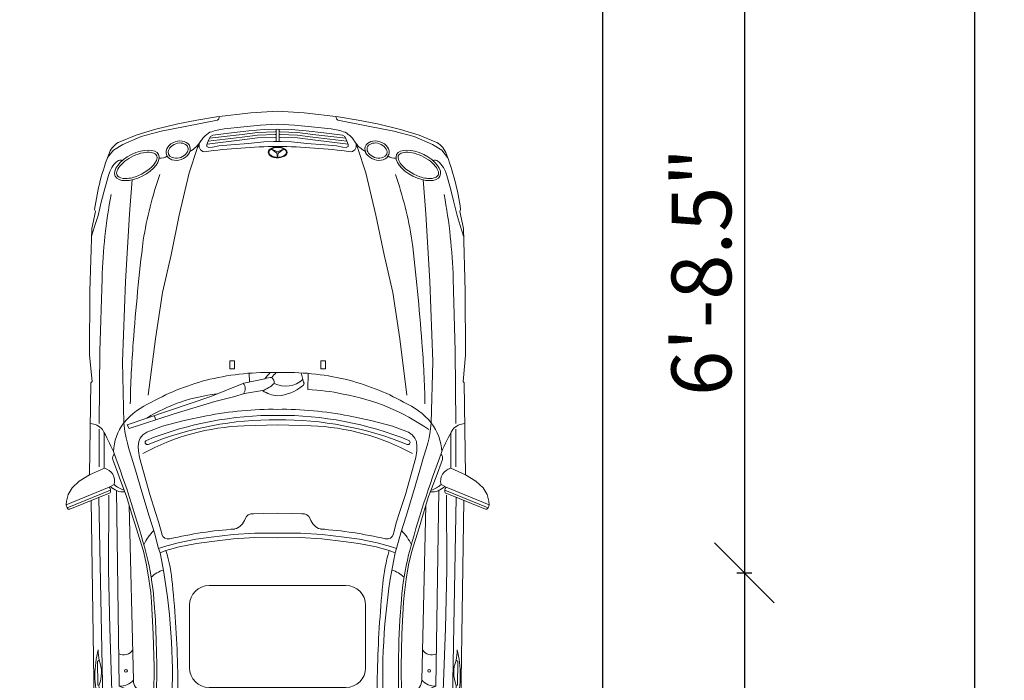
# Model space of a CAD drawing. Units: inches. Extents: x 2561 to 3163, y 493 to 1211.
# Tile 5 of 8: x 3031 to 3163, y 600 to 689. Entities that reach past the tile are written whole.
import ezdxf

# ---------------------------------------------------------------- set-up
doc = ezdxf.new("R2010")
doc.units = ezdxf.units.IN
for name, color, linetype, lineweight in [('0_Equip', 250, 'Continuous', 13), ('A-ANNO-DIMS', 2, 'Continuous', 18), ('A-SITE-PRKG', 8, 'Continuous', 25)]:
    doc.layers.add(name, color=color, linetype=linetype, lineweight=lineweight)
doc.styles.get("Standard").update_dxf_attribs({"font": 'arial.ttf'})
doc.dimstyles.new('ISO-25', dxfattribs={"dimtxt": 8, "dimasz": 8, "dimexe": 1, "dimexo": 1, "dimtad": 1, "dimlunit": 3, "dimtxsty": 'Standard', "dimblk": 'OBLIQUE', "dimcen": 2.5, "dimadec": 0, "dimazin": 0, "dimtfac": 1, "dimtmove": 0, "dimatfit": 3, "dimfxl": 1, "dimfxlon": 1, "dimarcsym": 0})

# ---------------------------------------------------------------- blocks, each defined once
blk = doc.blocks.new('A$C4C7B54D1')
at = {"layer": '0_Equip', "ltscale": 0.1}
for p, q in [((-1.0176, 2.6505), (-1.112, 2.6343)), ((-0.8531, 2.6707), (-1.0176, 2.6505)), ((-0.7257, 2.678), (-0.8531, 2.6707)), ((-0.7257, 2.678), (-0.5983, 2.6707)), ((-0.5983, 2.6707), (-0.4338, 2.6505)), ((-0.4338, 2.6505), (-0.3394, 2.6343)), ((-1.2037, 2.6168), (-1.3142, 2.5898)), ((-1.1673, 2.6045), (-1.2824, 2.5829)), ((-1.112, 2.6343), (-1.2037, 2.6168)), ((-1.0138, 2.6343), (-1.1673, 2.6045)), ((-0.8877, 2.6027), (-0.9812, 2.5937)), ((-0.8072, 2.6112), (-0.8877, 2.6027)), ((-0.7257, 2.6157), (-0.8072, 2.6112)), ((-0.7257, 2.6157), (-0.6441, 2.6112)), ((-0.6441, 2.6112), (-0.5636, 2.6027)), ((-0.5636, 2.6027), (-0.4701, 2.5937)), ((-0.4376, 2.6343), (-0.284, 2.6045)), ((-0.3394, 2.6343), (-0.2477, 2.6168)), ((-0.284, 2.6045), (-0.1689, 2.5829)), ((-0.2477, 2.6168), (-0.1371, 2.5898)), ((-1.4032, 2.5628), (-1.4801, 2.5318)), ((-1.3789, 2.557), (-1.4667, 2.5181)), ((-1.3142, 2.5898), (-1.4032, 2.5628)), ((-1.2824, 2.5829), (-1.3789, 2.557)), ((-0.1689, 2.5829), (-0.0725, 2.557)), ((-0.1371, 2.5898), (-0.0481, 2.5628)), ((-0.0725, 2.557), (0.0153, 2.5181)), ((-0.0481, 2.5628), (0.0288, 2.5318)), ((-1.4667, 2.5181), (-1.5113, 2.4907)), ((-1.1083, 2.5037), (-1.1486, 2.3827)), ((-0.343, 2.5037), (-0.3027, 2.3827)), ((0.0153, 2.5181), (0.06, 2.4907)), ((-1.5113, 2.4907), (-1.5393, 2.4562)), ((0.06, 2.4907), (0.0879, 2.4562)), ((-1.5353, 2.3701), (-1.5529, 2.308)), ((-1.1486, 2.3827), (-1.1961, 2.1797)), ((-0.3027, 2.3827), (-0.2552, 2.1797)), ((0.084, 2.3701), (0.1016, 2.308)), ((-1.435, 2.1869), (-1.4221, 2.3511)), ((-0.0163, 2.1869), (-0.0293, 2.3511)), ((-1.5529, 2.308), (-1.5677, 2.2486)), ((0.1016, 2.308), (0.1164, 2.2486)), ((-1.5677, 2.2486), (-1.5849, 2.1795)), ((0.1164, 2.2486), (0.1336, 2.1795)), ((-1.597, 2.1976), (-1.615, 2.1169)), ((-1.6012, 2.2082), (-1.597, 2.1976)), ((-1.5849, 2.1795), (-1.5997, 2.1304)), ((-1.4537, 1.863), (-1.435, 2.1869)), ((-1.1961, 2.1797), (-1.2349, 1.9911)), ((-0.2552, 2.1797), (-0.2164, 1.9911)), ((0.0024, 1.863), (-0.0163, 2.1869)), ((0.1336, 2.1795), (0.1484, 2.1304)), ((0.1499, 2.2082), (0.1457, 2.1976)), ((0.1457, 2.1976), (0.1637, 2.1169)), ((-1.5997, 2.1304), (-1.6161, 2.0798)), ((0.1484, 2.1304), (0.1647, 2.0798)), ((-1.615, 2.1169), (-1.6235, 1.8165)), ((0.1637, 2.1169), (0.1722, 1.8165)), ((-1.2349, 1.9911), (-1.2767, 1.8097)), ((-0.2164, 1.9911), (-0.1746, 1.8097)), ((-1.566, 1.8774), (-1.5761, 1.5304)), ((-1.4681, 1.48), (-1.4537, 1.863)), ((0.0168, 1.48), (0.0024, 1.863)), ((0.1147, 1.8774), (0.1247, 1.5304)), ((-1.6235, 1.8165), (-1.6256, 1.5098)), ((-1.2767, 1.8097), (-1.3098, 1.588)), ((-0.1746, 1.8097), (-0.1415, 1.588)), ((0.1722, 1.8165), (0.1743, 1.5098)), ((-1.3098, 1.588), (-1.3443, 1.3187)), ((-0.1415, 1.588), (-0.107, 1.3187)), ((-1.6256, 1.5098), (-1.6129, 1.3846)), ((-1.5761, 1.5304), (-1.5789, 1.1834)), ((0.1247, 1.5304), (0.1276, 1.1834)), ((0.1743, 1.5098), (0.1616, 1.3846)), ((-1.461, 1.1868), (-1.4681, 1.48)), ((-0.955, 1.4459), (-0.955, 1.4827)), ((-0.955, 1.4827), (-0.9321, 1.4827)), ((-0.9321, 1.4827), (-0.9321, 1.4459)), ((-0.5192, 1.4827), (-0.5192, 1.4459)), ((-0.4964, 1.4827), (-0.5192, 1.4827)), ((-0.4964, 1.4459), (-0.4964, 1.4827)), ((0.0097, 1.1868), (0.0168, 1.48)), ((-0.9321, 1.4459), (-0.955, 1.4459)), ((-0.8614, 1.4242), (-0.8603, 1.382)), ((-0.6135, 1.4258), (-0.6012, 1.3814)), ((-0.5809, 1.3459), (-0.5793, 1.4233)), ((-0.5192, 1.4459), (-0.4964, 1.4459)), ((-1.6193, 1.3782), (-1.6252, 0.9375)), ((-1.6129, 1.3846), (-1.6193, 1.3782)), ((-0.8878, 1.3764), (-1.0456, 1.313)), ((-0.7861, 1.3973), (-0.8878, 1.3764)), ((0.1616, 1.3846), (0.1679, 1.3782)), ((0.1679, 1.3782), (0.1739, 0.9375)), ((-0.9361, 1.3119), (-0.8835, 1.3269)), ((-0.8835, 1.3269), (-0.7975, 1.3408)), ((-1.0456, 1.313), (-1.4462, 1.1776)), ((-1.2207, 1.2292), (-1.0263, 1.2883)), ((-1.0263, 1.2883), (-0.9361, 1.3119)), ((-1.4366, 1.1604), (-1.2207, 1.2292)), ((-1.4565, 1.1447), (-1.461, 1.1868)), ((-1.3162, 1.2215), (-1.3088, 1.2011)), ((-1.1723, 1.1976), (-1.2762, 1.1716)), ((-1.0667, 1.22), (-1.1723, 1.1976)), ((-0.3847, 1.22), (-0.279, 1.1976)), ((-0.279, 1.1976), (-0.1751, 1.1716)), ((0.0052, 1.1447), (0.0097, 1.1868)), ((-1.5793, 1.1562), (-1.5793, 0.9761)), ((-1.5552, 1.139), (-1.5552, 0.9693)), ((-1.4503, 1.1151), (-1.4565, 1.1447)), ((-1.4462, 1.1776), (-1.4366, 1.1604)), ((-1.3515, 1.142), (-1.3703, 1.1286)), ((-1.2762, 1.1716), (-1.3515, 1.142)), ((-0.7257, 1.1776), (-0.8858, 1.1725)), ((-0.7257, 1.1776), (-0.5655, 1.1725)), ((-0.1751, 1.1716), (-0.0999, 1.142)), ((-0.0999, 1.142), (-0.0811, 1.1286)), ((-0.0011, 1.1151), (0.0052, 1.1447)), ((0.1038, 1.139), (0.1038, 0.9693)), ((0.128, 1.1562), (0.128, 0.9761)), ((-1.444, 1.0892), (-1.4503, 1.1151)), ((-1.4368, 1.0623), (-1.444, 1.0892)), ((-1.39, 1.0981), (-1.3927, 1.0739)), ((-1.3828, 1.1133), (-1.39, 1.0981)), ((-1.3703, 1.1286), (-1.3828, 1.1133)), ((-0.0811, 1.1286), (-0.0685, 1.1133)), ((-0.0685, 1.1133), (-0.0614, 1.0981)), ((-0.0614, 1.0981), (-0.0587, 1.0739)), ((-0.0145, 1.0623), (-0.0073, 1.0892)), ((-0.0073, 1.0892), (-0.0011, 1.1151)), ((-1.4243, 1.0229), (-1.4368, 1.0623)), ((-1.3927, 1.0739), (-1.3918, 1.0533)), ((-1.3918, 1.0533), (-1.3867, 1.0211)), ((-0.0596, 1.0533), (-0.0646, 1.0211)), ((-0.0587, 1.0739), (-0.0596, 1.0533)), ((-0.027, 1.0229), (-0.0145, 1.0623)), ((-1.5149, 1.011), (-1.4844, 0.9277)), ((-1.4064, 0.961), (-1.4243, 1.0229)), ((-1.3867, 1.0211), (-1.3374, 0.8446)), ((-0.0646, 1.0211), (-0.1139, 0.8446)), ((-0.0449, 0.961), (-0.027, 1.0229)), ((0.0635, 1.011), (0.0331, 0.9277)), ((-1.6252, 0.9375), (-1.5546, 0.9696)), ((-1.3759, 0.8562), (-1.4064, 0.961)), ((-0.0754, 0.8562), (-0.0449, 0.961)), ((0.1739, 0.9375), (0.1032, 0.9696)), ((-1.6745, 0.908), (-1.7088, 0.8764)), ((-1.6252, 0.9375), (-1.6745, 0.908)), ((-1.4844, 0.9277), (-1.4486, 0.8345)), ((0.0331, 0.9277), (-0.0028, 0.8345)), ((0.1739, 0.9375), (0.2232, 0.908)), ((0.2232, 0.908), (0.2574, 0.8764)), ((-1.5321, 0.8786), (-1.7381, 0.7945)), ((-1.5253, 0.865), (-1.7329, 0.7802)), ((-1.7088, 0.8764), (-1.728, 0.8432)), ((-1.5273, 0.8512), (-1.7203, 0.7738)), ((-1.508, 0.8914), (-1.5321, 0.8786)), ((-1.4835, -0.0735), (-1.497, 0.863)), ((-1.3401, 0.7406), (-1.3759, 0.8562)), ((-0.1112, 0.7406), (-0.0754, 0.8562)), ((0.0322, -0.0735), (0.0457, 0.863)), ((0.0566, 0.8914), (0.0807, 0.8786)), ((0.074, 0.865), (0.2816, 0.7802)), ((0.0759, 0.8512), (0.269, 0.7738)), ((0.0807, 0.8786), (0.2867, 0.7945)), ((0.2574, 0.8764), (0.2767, 0.8432)), ((-1.7366, 0.8127), (-1.7377, 0.7934)), ((-1.728, 0.8432), (-1.7366, 0.8127)), ((-1.6171, 0.8152), (-1.5964, -0.6171)), ((-1.5805, 0.8299), (-1.5623, -0.138)), ((-1.5337, 0.8406), (-1.5355, 0.484)), ((-1.4486, 0.8345), (-1.4226, 0.7503)), ((-1.3374, 0.8446), (-1.3097, 0.7577)), ((-0.1139, 0.8446), (-0.1417, 0.7577)), ((-0.0028, 0.8345), (-0.0287, 0.7503)), ((0.0824, 0.8406), (0.0842, 0.484)), ((0.1292, 0.8299), (0.111, -0.138)), ((0.1658, 0.8152), (0.145, -0.6171)), ((0.2767, 0.8432), (0.2853, 0.8127)), ((0.2853, 0.8127), (0.2863, 0.7934)), ((-1.7377, 0.7934), (-1.7327, 0.7794)), ((-1.4352, 0.792), (-1.4152, -0.045)), ((-1.3097, 0.7577), (-1.2953, 0.7129)), ((-0.7257, 0.7541), (-0.7926, 0.7532)), ((-0.7257, 0.7541), (-0.6587, 0.7532)), ((-0.1417, 0.7577), (-0.156, 0.7129)), ((-0.0162, 0.792), (-0.0361, -0.045)), ((0.2863, 0.7934), (0.2813, 0.7794)), ((-1.4226, 0.7503), (-1.4029, 0.6849)), ((-1.315, 0.66), (-1.3401, 0.7406)), ((-1.2953, 0.7129), (-1.2801, 0.6573)), ((-0.7926, 0.7532), (-0.8418, 0.7514)), ((-0.6587, 0.7532), (-0.6095, 0.7514)), ((-0.156, 0.7129), (-0.1712, 0.6573)), ((-0.1363, 0.66), (-0.1112, 0.7406)), ((-0.0287, 0.7503), (-0.0484, 0.6849)), ((-1.4029, 0.6849), (-1.368, 0.5729)), ((-1.2951, 0.5849), (-1.315, 0.66)), ((-0.1562, 0.5849), (-0.1363, 0.66)), ((-0.0484, 0.6849), (-0.0834, 0.5729)), ((-1.2801, 0.6573), (-1.2795, 0.6546)), ((-1.2021, 0.6133), (-1.2663, 0.5956)), ((-1.1177, 0.6302), (-1.2021, 0.6133)), ((-1.0437, 0.6403), (-1.1177, 0.6302)), ((-1.0411, 0.6196), (-1.1142, 0.6096)), ((-0.9389, 0.6526), (-1.0437, 0.6403)), ((-0.937, 0.6317), (-1.0411, 0.6196)), ((-0.8346, 0.6593), (-0.9389, 0.6526)), ((-0.834, 0.6384), (-0.937, 0.6317)), ((-0.7257, 0.6582), (-0.8346, 0.6593)), ((-0.7257, 0.6373), (-0.834, 0.6384)), ((-0.7257, 0.6582), (-0.6168, 0.6593)), ((-0.7257, 0.6373), (-0.6173, 0.6384)), ((-0.6173, 0.6384), (-0.5143, 0.6317)), ((-0.6168, 0.6593), (-0.5124, 0.6526)), ((-0.5143, 0.6317), (-0.4102, 0.6196)), ((-0.5124, 0.6526), (-0.4076, 0.6403)), ((-0.4102, 0.6196), (-0.3371, 0.6096)), ((-0.4076, 0.6403), (-0.3337, 0.6302)), ((-0.3337, 0.6302), (-0.2492, 0.6133)), ((-0.2492, 0.6133), (-0.185, 0.5956)), ((-0.1712, 0.6573), (-0.1719, 0.6546)), ((-1.368, 0.5729), (-1.3527, 0.5066)), ((-1.2663, 0.5956), (-1.2951, 0.5849)), ((-1.2879, 0.5653), (-1.2951, 0.5849)), ((-1.2599, 0.5757), (-1.2879, 0.5653)), ((-1.1973, 0.593), (-1.2599, 0.5757)), ((-1.1142, 0.6096), (-1.1973, 0.593)), ((-0.3371, 0.6096), (-0.2541, 0.593)), ((-0.2541, 0.593), (-0.1914, 0.5757)), ((-0.1914, 0.5757), (-0.1635, 0.5653)), ((-0.185, 0.5956), (-0.1562, 0.5849)), ((-0.1635, 0.5653), (-0.1562, 0.5849)), ((-0.0834, 0.5729), (-0.0986, 0.5066)), ((-1.5355, 0.484), (-1.5292, 0.2045)), ((-1.3527, 0.5066), (-1.3411, 0.4394)), ((-0.0986, 0.5066), (-0.1102, 0.4394)), ((0.0842, 0.484), (0.0779, 0.2045)), ((-1.3411, 0.4394), (-1.3321, 0.3749)), ((-0.1102, 0.4394), (-0.1192, 0.3749)), ((-0.7257, 0.4085), (-1.0528, 0.4085)), ((-0.7257, 0.4085), (-0.3986, 0.4085)), ((-1.3321, 0.3749), (-1.3286, 0.3301)), ((-1.3286, 0.3301), (-1.3204, 0.1751)), ((-1.3178, 0.3418), (-1.31, 0.2426)), ((-0.1335, 0.3418), (-0.1413, 0.2426)), ((-0.1228, 0.3301), (-0.1309, 0.1751)), ((-0.1192, 0.3749), (-0.1228, 0.3301)), ((-1.1468, 0.3145), (-1.1468, 0.0145)), ((-0.3045, 0.3145), (-0.3045, 0.0145)), ((-1.31, 0.2426), (-1.306, 0.1454)), ((-0.1413, 0.2426), (-0.1454, 0.1454)), ((-1.5292, 0.2045), (-1.5185, -0.0974)), ((0.0779, 0.2045), (0.0672, -0.0974)), ((-1.3204, 0.1751), (-1.3164, 0.0193)), ((-1.306, 0.1454), (-1.3036, 0.0305)), ((-0.1454, 0.1454), (-0.1478, 0.0305)), ((-0.1309, 0.1751), (-0.1349, 0.0193)), ((-1.5798, 0.0505), (-1.5879, 0.0456)), ((0.1285, 0.0505), (0.1365, 0.0456)), ((-1.5879, 0.0456), (-1.5863, -0.0676)), ((-1.3164, 0.0193), (-1.3178, -0.1112)), ((-1.3036, 0.0305), (-1.3044, -0.1358)), ((-0.1478, 0.0305), (-0.147, -0.1358)), ((-0.1349, 0.0193), (-0.1335, -0.1112)), ((0.1365, 0.0456), (0.1349, -0.0676)), ((-1.5863, -0.0676), (-1.5806, -0.0692)), ((-0.7257, -0.0796), (-1.0528, -0.0796)), ((-0.7257, -0.0796), (-0.3986, -0.0796)), ((0.1349, -0.0676), (0.1293, -0.0692)), ((-1.4948, -0.0965), (-1.5413, -0.143)), ((-1.5147, -0.1299), (-1.5058, -0.3725)), ((-1.4857, -0.1082), (-1.4866, -0.2223)), ((-1.3774, -0.0972), (-1.3178, -0.1112)), ((-0.0739, -0.0972), (-0.1335, -0.1112)), ((0.0344, -0.1082), (0.0352, -0.2223)), ((0.0435, -0.0965), (0.0899, -0.143)), ((0.0633, -0.1299), (0.0545, -0.3725)), ((-1.5413, -0.143), (-1.5686, -0.1663)), ((-1.4713, -0.1773), (-1.4737, -0.2127)), ((0.02, -0.1773), (0.0224, -0.2127)), ((0.0899, -0.143), (0.1172, -0.1663)), ((-1.4866, -0.2223), (-1.4809, -0.3653)), ((-1.4737, -0.2127), (-1.4705, -0.3187)), ((0.0224, -0.2127), (0.0192, -0.3187)), ((0.0352, -0.2223), (0.0296, -0.3653)), ((-1.3211, -0.2496), (-1.3332, -0.3629)), ((-0.1302, -0.2496), (-0.1182, -0.3629)), ((-1.4705, -0.3187), (-1.4649, -0.4424)), ((0.0192, -0.3187), (0.0135, -0.4424)), ((-1.5058, -0.3725), (-1.4922, -0.6007)), ((-1.4809, -0.3653), (-1.4745, -0.5203)), ((-1.3332, -0.3629), (-1.3516, -0.4906)), ((-0.1182, -0.3629), (-0.0997, -0.4906)), ((0.0296, -0.3653), (0.0232, -0.5203)), ((0.0545, -0.3725), (0.0408, -0.6007)), ((-1.4649, -0.4424), (-1.4576, -0.5822)), ((0.0135, -0.4424), (0.0063, -0.5822)), ((-1.3516, -0.4906), (-1.3725, -0.5902)), ((-0.0997, -0.4906), (-0.0788, -0.5902)), ((-1.4745, -0.5203), (-1.4665, -0.6617)), ((0.0232, -0.5203), (0.0151, -0.6617)), ((-1.4922, -0.6007), (-1.4712, -0.814)), ((-1.4576, -0.5822), (-1.4384, -0.7806)), ((-1.3725, -0.5902), (-1.3942, -0.6641)), ((-0.0788, -0.5902), (-0.0571, -0.6641)), ((0.0063, -0.5822), (-0.013, -0.7806)), ((0.0408, -0.6007), (0.0198, -0.814)), ((-1.5964, -0.6171), (-1.5863, -0.6228)), ((-1.5863, -0.6228), (-1.5949, -0.6885)), ((-1.3094, -0.9936), (-1.2569, -0.6398)), ((-0.1419, -0.9936), (-0.1944, -0.6398)), ((0.145, -0.6171), (0.1349, -0.6228)), ((0.1349, -0.6228), (0.1436, -0.6885)), ((-1.5949, -0.6885), (-1.605, -0.843)), ((-1.4665, -0.6617), (-1.4552, -0.7742)), ((-1.3942, -0.6641), (-1.4199, -0.7485)), ((-0.0571, -0.6641), (-0.0314, -0.7485)), ((0.0151, -0.6617), (0.0039, -0.7742)), ((0.1436, -0.6885), (0.1537, -0.843)), ((-1.4199, -0.7485), (-1.4384, -0.7806)), ((-1.2616, -0.7846), (-1.2511, -0.7134)), ((-0.1898, -0.7846), (-0.2003, -0.7134)), ((-0.0314, -0.7485), (-0.013, -0.7806)), ((-1.2826, -0.9445), (-1.2616, -0.7846)), ((-0.9336, -0.7717), (-0.7257, -0.7787)), ((-0.9331, -0.7613), (-0.7253, -0.7683)), ((-0.5182, -0.7613), (-0.726, -0.7683)), ((-0.5177, -0.7717), (-0.7257, -0.7787)), ((-0.1688, -0.9445), (-0.1898, -0.7846)), ((-1.605, -0.843), (-1.605, -1.0322)), ((0.1537, -0.843), (0.1537, -1.0322)), ((-1.3094, -1.1068), (-1.2826, -0.9445)), ((-0.1419, -1.1068), (-0.1688, -0.9445)), ((-1.605, -1.0322), (-1.592, -1.2661)), ((-1.3444, -1.2014), (-1.3094, -0.9936)), ((-0.1069, -1.2014), (-0.1419, -0.9936)), ((0.1537, -1.0322), (0.1407, -1.2661)), ((-1.3386, -1.2925), (-1.3094, -1.1068)), ((-0.1127, -1.2925), (-0.1419, -1.1068)), ((-1.565, -1.3405), (-1.592, -1.2661)), ((-1.592, -1.2661), (-1.5848, -1.3051)), ((0.1137, -1.3405), (0.1407, -1.2661)), ((0.1407, -1.2661), (0.1335, -1.3051)), ((-1.5848, -1.3051), (-1.5762, -1.4004)), ((-1.1985, -1.3182), (-1.1694, -1.3835)), ((-0.2528, -1.3182), (-0.282, -1.3835)), ((0.1335, -1.3051), (0.1248, -1.4004)), ((-1.5417, -1.4736), (-1.565, -1.3405)), ((-0.88, -1.3337), (-0.8328, -1.3271)), ((-0.8328, -1.3271), (-0.7257, -1.3271)), ((-0.6185, -1.3271), (-0.7257, -1.3271)), ((-0.5713, -1.3337), (-0.6185, -1.3271)), ((0.0904, -1.4736), (0.1137, -1.3405)), ((-1.5762, -1.4004), (-1.5486, -1.6107)), ((-1.0858, -1.3979), (-1.0181, -1.3979)), ((-0.8409, -1.4088), (-0.8488, -1.4158)), ((-0.8309, -1.402), (-0.8409, -1.4088)), ((-0.8163, -1.3979), (-0.8309, -1.402)), ((-0.7257, -1.3974), (-0.8163, -1.3979)), ((-0.7257, -1.3974), (-0.635, -1.3979)), ((-0.635, -1.3979), (-0.6204, -1.402)), ((-0.6204, -1.402), (-0.6104, -1.4088)), ((-0.6104, -1.4088), (-0.6025, -1.4158)), ((-0.3655, -1.3979), (-0.4333, -1.3979)), ((0.1248, -1.4004), (0.0973, -1.6107)), ((-1.0923, -1.4501), (-0.9989, -1.4699)), ((-0.8696, -1.4545), (-0.8731, -1.467)), ((-0.8664, -1.4423), (-0.8696, -1.4545)), ((-0.861, -1.4312), (-0.8664, -1.4423)), ((-0.8558, -1.4236), (-0.861, -1.4312)), ((-0.8488, -1.4158), (-0.8558, -1.4236)), ((-0.6025, -1.4158), (-0.5955, -1.4236)), ((-0.5955, -1.4236), (-0.5904, -1.4312)), ((-0.5904, -1.4312), (-0.585, -1.4423)), ((-0.585, -1.4423), (-0.5817, -1.4545)), ((-0.5817, -1.4545), (-0.5782, -1.467)), ((-0.359, -1.4501), (-0.4524, -1.4699)), ((-1.4962, -1.7129), (-1.5417, -1.4736)), ((-1.3456, -1.5004), (-1.3433, -1.7188)), ((-0.9989, -1.4699), (-0.8846, -1.4828)), ((-0.8807, -1.4821), (-0.8846, -1.4828)), ((-0.8846, -1.4828), (-0.8799, -1.5038)), ((-0.8769, -1.4791), (-0.8807, -1.4821)), ((-0.8799, -1.5038), (-0.8706, -1.5038)), ((-0.8745, -1.477), (-0.8769, -1.4791)), ((-0.8731, -1.467), (-0.8745, -1.477)), ((-0.7257, -1.4865), (-0.8374, -1.4884)), ((-0.7257, -1.4969), (-0.837, -1.4988)), ((-0.7257, -1.4865), (-0.6139, -1.4884)), ((-0.7257, -1.4969), (-0.6143, -1.4988)), ((-0.5714, -1.5038), (-0.5808, -1.5038)), ((-0.5782, -1.467), (-0.5768, -1.477)), ((-0.5768, -1.477), (-0.5744, -1.4791)), ((-0.5744, -1.4791), (-0.5706, -1.4821)), ((-0.5668, -1.4828), (-0.5714, -1.5038)), ((-0.5706, -1.4821), (-0.5668, -1.4828)), ((-0.4524, -1.4699), (-0.5668, -1.4828)), ((-0.1057, -1.5004), (-0.1081, -1.7188)), ((0.0448, -1.7129), (0.0904, -1.4736)), ((-0.8799, -1.5352), (-0.7257, -1.5393)), ((-0.5714, -1.5352), (-0.7257, -1.5393)), ((-0.8502, -1.5951), (-0.7257, -1.5951)), ((-0.6011, -1.5951), (-0.7257, -1.5951)), ((-1.5486, -1.6107), (-1.5024, -1.8663)), ((-0.8507, -1.616), (-0.7257, -1.616)), ((-0.6006, -1.616), (-0.7257, -1.616)), ((0.0973, -1.6107), (0.0511, -1.8663)), ((-1.4584, -1.8701), (-1.4962, -1.7129)), ((-1.3433, -1.7188), (-1.3304, -1.8962)), ((-0.1081, -1.7188), (-0.1209, -1.8962)), ((0.0071, -1.8701), (0.0448, -1.7129)), ((-1.5024, -1.8663), (-1.4894, -1.914)), ((0.0511, -1.8663), (0.0381, -1.914)), ((-1.2767, -1.9721), (-1.3526, -1.9616)), ((-1.1845, -1.9838), (-1.2767, -1.9721)), ((-1.055, -1.9768), (-1.055, -1.9908)), ((-0.7257, -1.985), (-1.055, -1.9768)), ((-0.7257, -1.985), (-0.3964, -1.9768)), ((-0.3964, -1.9768), (-0.3964, -1.9908)), ((-0.2668, -1.9838), (-0.1746, -1.9721)), ((-0.1746, -1.9721), (-0.0987, -1.9616)), ((-1.3797, -2.0208), (-1.1314, -2.0483)), ((-1.055, -1.9908), (-1.1845, -1.9838)), ((-0.9663, -2.0048), (-0.7257, -2.0048)), ((-0.4851, -2.0048), (-0.7257, -2.0048)), ((-0.3964, -1.9908), (-0.2668, -1.9838)), ((-0.0716, -2.0208), (-0.3199, -2.0483)), ((-1.1314, -2.0483), (-0.8803, -2.0598)), ((-1.0585, -2.0375), (-0.9383, -2.0469)), ((-0.9383, -2.0469), (-0.7784, -2.0504)), ((-0.8803, -2.0598), (-0.7257, -2.0598)), ((-0.7784, -2.0504), (-0.7257, -2.0504)), ((-0.673, -2.0504), (-0.7257, -2.0504)), ((-0.5711, -2.0598), (-0.7257, -2.0598)), ((-0.5131, -2.0469), (-0.673, -2.0504)), ((-0.3199, -2.0483), (-0.5711, -2.0598)), ((-0.3929, -2.0375), (-0.5131, -2.0469))]:
    blk.add_line(p, q, dxfattribs=at)
at = {"layer": '0_Equip'}
for p, q in [((-0.7257, 2.5926), (-0.7905, 2.5897)), ((-0.733, 2.5923), (-0.733, 2.5325)), ((-0.7257, 2.5926), (-0.6608, 2.5897)), ((-0.7183, 2.5923), (-0.7183, 2.5325)), ((-1.0577, 2.5343), (-0.8949, 2.5537)), ((-1.0475, 2.557), (-1.0545, 2.5425)), ((-1.0517, 2.5482), (-0.8949, 2.567)), ((-1.0364, 2.5634), (-1.0475, 2.557)), ((-0.9467, 2.5739), (-1.0364, 2.5634)), ((-0.8628, 2.5838), (-0.9467, 2.5739)), ((-0.8949, 2.567), (-0.8211, 2.5763)), ((-0.8949, 2.5537), (-0.8211, 2.5631)), ((-0.8949, 2.5405), (-0.8211, 2.5498)), ((-0.7905, 2.5897), (-0.8628, 2.5838)), ((-0.8211, 2.5763), (-0.738, 2.5791)), ((-0.8211, 2.5631), (-0.738, 2.5659)), ((-0.8211, 2.5498), (-0.738, 2.5526)), ((-0.738, 2.5791), (-0.733, 2.58)), ((-0.738, 2.5659), (-0.733, 2.5668)), ((-0.738, 2.5526), (-0.733, 2.5536)), ((-0.7133, 2.5791), (-0.7183, 2.58)), ((-0.7133, 2.5659), (-0.7183, 2.5668)), ((-0.7133, 2.5526), (-0.7183, 2.5536)), ((-0.6302, 2.5763), (-0.7133, 2.5791)), ((-0.6302, 2.5631), (-0.7133, 2.5659)), ((-0.6302, 2.5498), (-0.7133, 2.5526)), ((-0.6608, 2.5897), (-0.5886, 2.5838)), ((-0.5564, 2.567), (-0.6302, 2.5763)), ((-0.5564, 2.5537), (-0.6302, 2.5631)), ((-0.5564, 2.5405), (-0.6302, 2.5498)), ((-0.5886, 2.5838), (-0.5046, 2.5739)), ((-0.3996, 2.5482), (-0.5564, 2.567)), ((-0.3936, 2.5343), (-0.5564, 2.5537)), ((-0.5046, 2.5739), (-0.4149, 2.5634)), ((-0.4149, 2.5634), (-0.4038, 2.557)), ((-0.4038, 2.557), (-0.3968, 2.5425)), ((-1.0545, 2.5425), (-1.0638, 2.5185)), ((-1.0638, 2.5185), (-1.0638, 2.5092)), ((-1.0638, 2.5092), (-1.0545, 2.504)), ((-1.0631, 2.5204), (-0.8949, 2.5405)), ((-1.0545, 2.504), (-1.0376, 2.5051)), ((-1.0376, 2.5051), (-1.0067, 2.5116)), ((-1.0067, 2.5116), (-0.9502, 2.5168)), ((-0.9502, 2.5168), (-0.8657, 2.5238)), ((-0.8657, 2.5238), (-0.7922, 2.5308)), ((-0.7922, 2.5308), (-0.7433, 2.5325)), ((-0.7433, 2.5325), (-0.7257, 2.5325)), ((-0.7389, 2.5095), (-0.7395, 2.5059)), ((-0.6947, 2.4974), (-0.7261, 2.4828)), ((-0.708, 2.5325), (-0.7257, 2.5325)), ((-0.6947, 2.4974), (-0.723, 2.4776)), ((-0.7124, 2.5095), (-0.7119, 2.5059)), ((-0.6591, 2.5308), (-0.708, 2.5325)), ((-0.5857, 2.5238), (-0.6591, 2.5308)), ((-0.5011, 2.5168), (-0.5857, 2.5238)), ((-0.3882, 2.5204), (-0.5564, 2.5405)), ((-0.4446, 2.5116), (-0.5011, 2.5168)), ((-0.4137, 2.5051), (-0.4446, 2.5116)), ((-0.3968, 2.504), (-0.4137, 2.5051)), ((-0.3968, 2.5425), (-0.3875, 2.5185)), ((-0.3875, 2.5092), (-0.3968, 2.504)), ((-0.3875, 2.5185), (-0.3875, 2.5092)), ((-0.7566, 2.4971), (-0.7261, 2.4828)), ((-0.7566, 2.4971), (-0.7291, 2.4776)), ((-0.7259, 2.4578), (-0.7291, 2.4776)), ((-0.7259, 2.4578), (-0.723, 2.4776))]:
    blk.add_line(p, q, dxfattribs=at)
at = {"layer": '0_Equip', "ltscale": 0.1}
for centre in [(-1.4513, 0), (0, 0)]:
    blk.add_circle(centre, 0.00662, dxfattribs=at)
for centre, radius, start, end in [((-1.0252, 2.6508), 0.02, 304.7228, 3.5172), ((-0.4261, 2.6508), 0.02, 176.4828, 235.2772), ((-0.9299, 2.2354), 0.3619, 98.1466, 109.2524), ((-0.5214, 2.2354), 0.3619, 70.7476, 81.8534), ((-0.9799, 2.461), 0.1353, 120.8369, 151.2853), ((-0.4714, 2.461), 0.1353, 28.7147, 59.1631), ((-1.4391, 2.4422), 0.0986, 114.5945, 157.5113), ((-1.2153, 2.6098), 0.1432, 299.1564, 328.1831), ((-0.9799, 2.461), 0.1353, 151.2853, 161.5889), ((-1.0728, 2.5126), 0.029, 152.6038, 261.721), ((-0.6679, -0.6671), 3.1773, 91.0415, 97.3969), ((-0.7834, -0.6671), 3.1773, 82.6031, 88.9585), ((-0.3785, 2.5126), 0.029, 278.279, 27.3962), ((-0.236, 2.6098), 0.1432, 211.8169, 240.8436), ((-0.4714, 2.461), 0.1353, 18.4111, 28.7147), ((-0.0123, 2.4422), 0.0986, 22.4887, 65.4055), ((-0.4722, 2.0579), 1.139, 158.2564, 172.4203), ((-1.2841, 2.5028), 0.0501, 260.5448, 306.7068), ((-0.1672, 2.5028), 0.0501, 233.2932, 279.4552), ((-0.9791, 2.0579), 1.139, 7.5797, 21.7436), ((-1.4083, 2.3394), 0.1306, 130.2084, 166.4224), ((-1.4798, 2.4259), 0.0184, 54.8052, 134.0204), ((0.0285, 2.4259), 0.0184, 45.9796, 125.1948), ((-0.043, 2.3394), 0.1306, 13.5776, 49.7916), ((0.5502, 1.746), 1.9445, 161.1117, 170.7019), ((-2.0015, 1.746), 1.9445, 9.2981, 18.8883), ((1.1202, 1.7918), 2.6875, 169.5541, 178.1755), ((-2.5715, 1.7918), 2.6875, 1.8245, 10.4459), ((9.2655, 0.7813), 10.7109, 173.14258, 175.77374), ((-10.7169, 0.7813), 10.7109, 4.22626, 6.85742), ((2.9623, 1.2089), 4.3935, 175.2767, 179.1124), ((-4.4136, 1.2089), 4.3935, 0.8876, 4.7233), ((-0.7686, 0.201), 1.2267, 87.9955, 103.2364), ((-0.3726, 1.0935), 0.5131, 139.3585, 143.6922), ((-0.6528, 1.3354), 0.1211, 130.7679, 145.6911), ((-0.6828, 0.201), 1.2267, 76.7636, 92.0045), ((-0.786, 0.3109), 1.1158, 103.6551, 119.1148), ((-0.9216, 1.3498), 0.0409, 323.4512, 39.0343), ((-0.8494, 1.486), 0.1542, 289.6676, 314.192), ((-0.7554, 1.327), 0.0768, 88.1186, 113.6019), ((-0.7803, 1.3768), 0.0384, 357.9275, 44.3829), ((-0.6872, 1.4869), 0.1241, 243.8649, 311.6638), ((-0.6113, 1.3746), 0.0122, 294.8678, 33.6398), ((-0.6653, 0.3109), 1.1158, 60.8852, 76.3449), ((-0.929, 0.5266), 0.803, 96.22, 121.6991), ((-0.7147, 1.4628), 0.1474, 235.8143, 265.7174), ((-0.741, 1.5272), 0.212, 274.1513, 309.4931), ((-0.617, 0.3882), 0.9584, 77.6919, 87.8428), ((-0.5976, 0.2949), 1.0461, 55.3038, 79.8165), ((-1.1803, 0.9494), 0.3676, 113.8511, 139.7847), ((-0.2711, 0.9494), 0.3676, 40.2153, 66.1489), ((-0.7478, -0.378), 1.6295, 89.2231, 101.2856), ((-0.7036, -0.378), 1.6295, 78.7144, 90.7769), ((-1.6261, 1.102), 0.0813, 40.278, 87.0689), ((-1.2706, 1.0395), 0.2408, 142.2718, 177.7746), ((-0.7356, -0.4312), 1.6538, 89.6554, 111.9286), ((-0.7356, -0.4312), 1.6329, 89.6554, 111.9286), ((-0.7157, -0.4312), 1.6538, 68.0714, 90.3446), ((-0.7157, -0.4312), 1.6329, 68.0714, 90.3446), ((-0.1807, 1.0395), 0.2408, 2.2254, 37.7282), ((0.1747, 1.102), 0.0813, 92.9311, 139.722), ((-2.3477, 0.6968), 0.9076, 22.824, 30.2904), ((-0.85, 0.0855), 1.0875, 91.8892, 118.6013), ((-0.6014, 0.0855), 1.0875, 61.3987, 88.1108), ((0.8964, 0.6968), 0.9076, 149.7096, 157.176), ((-1.3493, 1.0932), 0.0105, 111.9286, 291.9286), ((-0.102, 1.0932), 0.0105, 248.0714, 68.0714), ((-1.4887, 1.0171), 0.0269, 132.3277, 193.1064), ((-6.6059, -0.8606), 5.4408, 15.0904, 20.5451), ((5.1546, -0.8606), 5.4408, 159.4549, 164.9096), ((0.0373, 1.0171), 0.0269, 346.8936, 47.6723), ((-1.5684, 0.9084), 0.0628, 344.3283, 77.2348), ((0.1171, 0.9084), 0.0628, 102.7652, 195.6717), ((-1.5495, 0.8614), 0.0245, 335.4987, 44.5114), ((-1.463, 0.9441), 0.0879, 224.7932, 273.9292), ((-1.4233, 0.9849), 0.1262, 227.8287, 253.081), ((0.0117, 0.9441), 0.0879, 266.0708, 315.2068), ((-0.0281, 0.9849), 0.1262, 286.919, 312.1713), ((0.0982, 0.8614), 0.0245, 135.4886, 204.5013), ((-1.7238, 0.7825), 0.00941, 199.646, 291.8616), ((0.2725, 0.7825), 0.00941, 248.1384, 340.354), ((-0.9515, 0.7495), 0.0737, 286.567, 342.4011), ((-0.8474, 0.7163), 0.0355, 80.937, 162.15), ((-0.6039, 0.7163), 0.0355, 17.85, 99.063), ((-0.4998, 0.7495), 0.0737, 197.5989, 253.433), ((-1.1535, 0.5061), 0.2334, 134.9877, 155.4049), ((-0.7896, -1.2957), 1.9795, 94.0807, 103.2045), ((-0.6617, -1.2957), 1.9795, 76.7955, 85.9193), ((-0.2978, 0.5061), 0.2334, 24.5951, 45.0123), ((-1.249, 0.662), 0.0314, 193.667, 283.2045), ((-0.2023, 0.662), 0.0314, 256.7955, 346.333), ((-2.0025, 0.3511), 0.7759, 4.7259, 16.8296), ((0.5512, 0.3511), 0.7759, 163.1704, 175.2741), ((-2.6334, 0.2371), 1.3197, 4.5498, 13.9797), ((-4.2099, -0.0242), 2.9809, 358.1905, 11.4064), ((2.7585, -0.0242), 2.9809, 168.5936, 181.8095), ((1.1821, 0.2371), 1.3197, 166.0203, 175.4502), ((-1.2324, 0.3484), 0.1397, 106.6168, 134.6647), ((-0.2189, 0.3484), 0.1397, 45.3353, 73.3832), ((-6.5594, -0.126), 5.3575, 1.3159, 5.7952), ((-1.0528, 0.3145), 0.0941, 90, 180), ((-0.3986, 0.3145), 0.0941, 0, 90), ((5.1081, -0.126), 5.3575, 174.2048, 178.6841), ((-1.0944, -0.0222), 0.5055, 165.8807, 194.1193), ((-1.3066, 0.102), 0.2781, 180.1936, 190.6834), ((-1.4634, 0.1296), 0.0534, 245.2796, 326.9469), ((0.0121, 0.1296), 0.0534, 213.0531, 294.7204), ((-0.1448, 0.102), 0.2781, 349.3166, 359.8064), ((-0.3569, -0.0222), 0.5055, 345.8807, 14.1193), ((-1.7275, -0.0084), 0.159, 337.4976, 21.7335), ((0.2762, -0.0084), 0.159, 158.2665, 202.5024), ((-1.0528, 0.0145), 0.0941, 180, 270), ((-0.3986, 0.0145), 0.0941, 270, 0), ((-1.4831, 0.0214), 0.095, 269.7172, 315.6185), ((-1.3634, -0.0473), 0.0519, 177.4537, 254.2676), ((-6.573, -0.0941), 5.3705, 356.0501, 0.9723), ((5.1217, -0.0941), 5.3705, 179.0277, 183.9499), ((-0.0879, -0.0473), 0.0519, 285.7324, 2.5463), ((0.0317, 0.0214), 0.095, 224.3815, 270.2828), ((-1.7817, -0.0969), 0.2029, 346.1346, 7.8419), ((-1.4874, -0.1039), 0.0105, 68.8598, 135.0096), ((-1.2476, 0.5164), 0.6547, 248.8598, 265.0222), ((-1.2968, 0.3651), 0.4767, 246.9385, 267.4714), ((-0.2038, 0.5164), 0.6547, 274.9778, 291.1402), ((-0.1545, 0.3651), 0.4767, 272.5286, 293.0615), ((0.0361, -0.1039), 0.0105, 44.9904, 111.1402), ((0.3303, -0.0969), 0.2029, 172.1581, 193.8654), ((-8.0298, -0.0355), 6.7998, 354.90123, 359.30214), ((6.5785, -0.0355), 6.7998, 180.69786, 185.09877), ((-1.5869, -0.1514), 0.0236, 227.2909, 320.7388), ((-1.3362, 0.3542), 0.5484, 255.7347, 268.4072), ((-0.1152, 0.3542), 0.5484, 271.5928, 284.2653), ((0.1355, -0.1514), 0.0236, 219.2612, 312.7091), ((-1.3699, -0.2402), 0.0497, 349.0381, 68.1064), ((-1.3526, -0.2358), 0.0418, 357.143, 88.4072), ((-0.0988, -0.2358), 0.0418, 91.5928, 182.857), ((-0.0814, -0.2402), 0.0497, 111.8936, 190.9619), ((-3.2483, -0.1412), 1.9399, 339.54, 357.143), ((1.797, -0.1412), 1.9399, 182.857, 200.46), ((-2.454, -0.4173), 1.2396, 346.6558, 357.8401), ((1.0027, -0.4173), 1.2396, 182.1599, 193.3442), ((-0.8588, 0.5276), 1.291, 252.4566, 266.6988), ((-0.5926, 0.5276), 1.291, 273.3012, 287.5434), ((-0.8588, 0.5276), 1.3014, 252.4566, 266.7043), ((-0.5926, 0.5276), 1.3014, 273.2957, 287.5434), ((-5.088, -0.3237), 3.9082, 348.7726, 353.1671), ((-1.1971, -0.7899), 0.0105, 79.1189, 173.1671), ((-0.7142, 1.7227), 2.5481, 259.1189, 269.7413), ((-0.7372, 1.7227), 2.5481, 270.2587, 280.8811), ((-0.2542, -0.7899), 0.0105, 6.8329, 100.8811), ((3.6366, -0.3237), 3.9082, 186.8329, 191.2274), ((-1.4504, -0.812), 0.0209, 185.6259, 339.54), ((-0.001, -0.812), 0.0209, 200.46, 354.3741), ((0.625, -1.1812), 0.5281, 165.7822, 187.813), ((0.1224, -1.0639), 0.0155, 11.61, 127.0083), ((-0.7003, -1.1122), 0.8395, 350.5693, 3.5107), ((-4.7286, -0.6026), 3.5073, 348.8701, 352.1003), ((3.2772, -0.6026), 3.5073, 187.8997, 191.1299), ((-0.8187, -1.3185), 0.5386, 167.4447, 180.7102), ((-0.6326, -1.3185), 0.5386, 359.2898, 12.5553), ((-1.3591, -1.3822), 0.1728, 21.7432, 61.9432), ((-0.0922, -1.3822), 0.1728, 118.0568, 158.2568), ((0.1138, -1.243), 0.0156, 219.7819, 334.4738), ((-1.0611, -1.2979), 0.2775, 178.8811, 209.7062), ((-1.0952, -1.3051), 0.1937, 172.4314, 224.4267), ((-0.3561, -1.3051), 0.1937, 315.5733, 7.5686), ((-0.3902, -1.2979), 0.2775, 330.2938, 1.1189), ((-1.0944, -1.3104), 0.2633, 183.2136, 211.504), ((-1.0482, -1.2146), 0.1871, 220.4031, 258.3959), ((-1.0495, -1.2507), 0.1505, 282.0448, 314.7653), ((-0.8301, -1.5634), 0.235, 102.268, 118.8572), ((-0.6213, -1.5634), 0.235, 61.1428, 77.732), ((-0.4019, -1.2507), 0.1505, 225.2347, 257.9552), ((-0.4032, -1.2146), 0.1871, 281.6041, 319.5969), ((-0.3569, -1.3104), 0.2633, 328.496, 356.7864), ((-1.0421, -1.3141), 0.145, 208.6187, 249.7318), ((-0.4092, -1.3141), 0.145, 290.2682, 331.3813), ((-1.2501, -1.516), 0.0967, 135.2951, 170.7274), ((-1.052, -1.2472), 0.3339, 216.9484, 253.2314), ((-1.052, -1.2472), 0.313, 216.9484, 253.2054), ((-0.8912, -0.9022), 0.6331, 235.8724, 271.0227), ((-1.0459, -1.2776), 0.2487, 221.0065, 261.6946), ((-0.5601, -0.9022), 0.6331, 268.9773, 304.1276), ((-0.4054, -1.2776), 0.2487, 278.3054, 318.9935), ((-0.3993, -1.2472), 0.313, 286.7946, 323.0516), ((-0.3993, -1.2472), 0.3339, 286.7686, 323.0516), ((-0.2012, -1.516), 0.0967, 9.2726, 44.7049), ((-0.8066, -1.54), 0.0735, 150.5285, 176.2825), ((-0.8344, -1.538), 0.0498, 93.4455, 136.5439), ((-0.8344, -1.538), 0.0393, 93.7549, 134.7116), ((-0.6169, -1.538), 0.0393, 45.2884, 86.2451), ((-0.6169, -1.538), 0.0498, 43.4561, 86.5545), ((-0.6447, -1.54), 0.0735, 3.7175, 29.4715), ((-0.7884, -0.3101), 1.2865, 254.0263, 267.246), ((-0.7003, 0.2815), 1.8451, 258.0669, 269.2129), ((-0.8066, -1.54), 0.063, 151.7195, 175.9212), ((-0.751, 0.2815), 1.8451, 270.7871, 281.9331), ((-0.6629, -0.3101), 1.2865, 272.754, 285.9737), ((-0.6447, -1.54), 0.063, 4.0788, 28.2805), ((-0.7884, -0.3101), 1.3074, 254.0198, 267.2681), ((-0.6629, -0.3101), 1.3074, 272.7319, 285.9802), ((-1.3393, -1.8393), 0.123, 194.4986, 263.7836), ((-0.1121, -1.8393), 0.123, 276.2164, 345.5014), ((-1.3628, -1.8937), 0.1282, 189.093, 262.4153), ((-0.5134, 7.9307), 9.8503, 265.23745, 268.76503), ((-1.2452, -1.8915), 0.0853, 183.2055, 252.6405), ((-0.938, 7.9307), 9.8503, 271.23497, 274.76255), ((-0.2061, -1.8915), 0.0853, 287.3595, 356.7945), ((-0.0885, -1.8937), 0.1282, 277.5847, 350.907), ((-1.0413, -1.8225), 0.2157, 228.406, 265.4391), ((-0.896, -1.272), 0.7362, 257.5275, 264.5209), ((-0.5554, -1.272), 0.7362, 275.4791, 282.4725), ((-0.41, -1.8225), 0.2157, 274.5609, 311.594)]:
    blk.add_arc(centre, radius, start, end, dxfattribs=at)
for centre, major_axis, ratio in [((-1.399, 2.4187), (-0.1036, -0.0518), 0.497493), ((-1.2016, 2.4892), (0.0562, 0.0189), 0.759763)]:
    blk.add_ellipse(centre, major_axis=major_axis, ratio=ratio, dxfattribs=at)
at = {"layer": '0_Equip'}
blk.add_ellipse((-0.7253, 2.4812), major_axis=(-0.0426, 0), ratio=0.550187, dxfattribs=at)
at = {"layer": '0_Equip', "ltscale": 0.1, "extrusion": (0, 0, -1)}
for centre, major_axis, ratio in [((-0.2497, 2.4892), (-0.0562, 0.0189), 0.759763), ((-0.0523, 2.4187), (0.1036, -0.0518), 0.497493)]:
    blk.add_ellipse(centre, major_axis=major_axis, ratio=ratio, dxfattribs=at)
at = {"layer": '0_Equip', "ltscale": 0.1}
for points, knots in [([(-1.1548, 2.5048), (-1.1596, 2.5191), (-1.1811, 2.5294), (-1.2283, 2.5198), (-1.248, 2.5001), (-1.2511, 2.4679), (-1.2373, 2.4539), (-1.1922, 2.4512), (-1.1656, 2.4658), (-1.1532, 2.4906), (-1.1526, 2.4983), (-1.1548, 2.5048)], [0, 0, 0, 0, 1.408119, 1.408119, 2.816238, 2.816238, 4.224358, 4.224358, 5.632477, 5.632477, 6.283185, 6.283185, 6.283185, 6.283185]), ([(-0.2965, 2.5048), (-0.2917, 2.5191), (-0.2703, 2.5294), (-0.2231, 2.5198), (-0.2033, 2.5001), (-0.2003, 2.4679), (-0.2141, 2.4539), (-0.2592, 2.4512), (-0.2858, 2.4658), (-0.2981, 2.4906), (-0.2987, 2.4983), (-0.2965, 2.5048)], [0, 0, 0, 0, 1.408119, 1.408119, 2.816238, 2.816238, 4.224358, 4.224358, 5.632477, 5.632477, 6.283185, 6.283185, 6.283185, 6.283185]), ([(-1.4937, 2.3714), (-1.4901, 2.3641), (-1.4809, 2.3581), (-1.4492, 2.3543), (-1.4277, 2.3571), (-1.3679, 2.3771), (-1.3298, 2.404), (-1.2994, 2.4483), (-1.2993, 2.4626), (-1.3171, 2.4801), (-1.3406, 2.4849), (-1.3989, 2.4733), (-1.4323, 2.4577), (-1.4816, 2.4186), (-1.4956, 2.3954), (-1.4959, 2.3774), (-1.4951, 2.3742), (-1.4937, 2.3714)], [0, 0, 0, 0, 0.646556, 0.646556, 1.293113, 1.293113, 2.410172, 2.410172, 3.309931, 3.309931, 4.20969, 4.20969, 5.109449, 5.109449, 6.031285, 6.031285, 6.283185, 6.283185, 6.283185, 6.283185]), ([(0.0424, 2.3714), (0.0388, 2.3641), (0.0295, 2.3581), (-0.0022, 2.3543), (-0.0236, 2.3571), (-0.0834, 2.3771), (-0.1216, 2.404), (-0.152, 2.4483), (-0.152, 2.4626), (-0.1343, 2.4801), (-0.1108, 2.4849), (-0.0524, 2.4733), (-0.019, 2.4577), (0.0303, 2.4186), (0.0443, 2.3954), (0.0445, 2.3774), (0.0438, 2.3742), (0.0424, 2.3714)], [0, 0, 0, 0, 0.646556, 0.646556, 1.293113, 1.293113, 2.410172, 2.410172, 3.309931, 3.309931, 4.20969, 4.20969, 5.109449, 5.109449, 6.031285, 6.031285, 6.283185, 6.283185, 6.283185, 6.283185])]:
    blk.add_open_spline(points, degree=3, knots=knots, dxfattribs=at)
at = {"layer": '0_Equip'}
blk.add_open_spline([(-0.7708, 2.4812), (-0.7708, 2.4725), (-0.7635, 2.4648), (-0.7294, 2.4499), (-0.6897, 2.4563), (-0.6733, 2.4916), (-0.7036, 2.5102), (-0.7526, 2.5051), (-0.7708, 2.4948), (-0.7708, 2.4812)], degree=3, knots=[0, 0, 0, 0, 0.903923, 0.903923, 2.878844, 2.878844, 4.872977, 4.872977, 6.283185, 6.283185, 6.283185, 6.283185], dxfattribs=at)
blk = doc.blocks.new('_Oblique')
at = {"color": 0, "linetype": 'ByBlock', "lineweight": -2}
blk.add_line((-0.5, -0.5), (0.5, 0.5), dxfattribs=at)
blk = doc.blocks.new('*D11')
at = {"layer": 'A-ANNO-DIMS', "color": 0, "lineweight": -2, "transparency": 16777216}
for p, q in [((3127.21, 695.07), (3129.21, 695.07)), ((3128.21, 695.07), (3128.21, 614.57)), ((3127.21, 614.57), (3129.21, 614.57))]:
    blk.add_line(p, q, dxfattribs=at)
at = {"layer": 'Defpoints', "color": 0, "transparency": 16777216}
for p in [(3109.27, 695.07), (2965.27, 614.57), (3128.21, 614.57)]:
    blk.add_point(p, dxfattribs=at)
at = {"layer": 'A-ANNO-DIMS', "color": 0, "lineweight": -2, "transparency": 16777216, "xscale": 8, "yscale": 8, "zscale": 8}
for p, rotation in [((3128.21, 695.07), 90), ((3128.21, 614.57), 270)]:
    blk.add_blockref('_Oblique', p, dxfattribs=dict(at, rotation=rotation))
at = {"layer": 'A-ANNO-DIMS', "color": 0, "transparency": 16777216, "insert": (3123.5, 654.82), "char_height": 8, "attachment_point": 5, "rotation": 90}
blk.add_mtext('6\'-8.5"', dxfattribs=at)
blk = doc.blocks.new('*D12')
at = {"layer": 'A-ANNO-DIMS', "color": 0, "lineweight": -2, "transparency": 16777216}
for p, q in [((3127.21, 614.57), (3129.21, 614.57)), ((3128.21, 614.57), (3128.21, 529.07)), ((3127.21, 529.07), (3129.21, 529.07))]:
    blk.add_line(p, q, dxfattribs=at)
at = {"layer": 'Defpoints', "color": 0, "transparency": 16777216}
for p in [(2965.27, 614.57), (2965.27, 529.07), (3128.21, 529.07)]:
    blk.add_point(p, dxfattribs=at)
at = {"layer": 'A-ANNO-DIMS', "color": 0, "lineweight": -2, "transparency": 16777216, "xscale": 8, "yscale": 8, "zscale": 8}
for p, rotation in [((3128.21, 614.57), 90), ((3128.21, 529.07), 270)]:
    blk.add_blockref('_Oblique', p, dxfattribs=dict(at, rotation=rotation))
at = {"layer": 'A-ANNO-DIMS', "color": 0, "transparency": 16777216, "insert": (3123.5, 571.82), "char_height": 8, "attachment_point": 5, "rotation": 90}
blk.add_mtext('7\'-1.5"', dxfattribs=at)
blk = doc.blocks.new('*D13')
at = {"layer": 'A-ANNO-DIMS', "color": 0, "lineweight": -2, "transparency": 16777216}
for p, q in [((3157.99, 1093.07), (3159.99, 1093.07)), ((3158.99, 1093.07), (3158.99, 529.07)), ((3157.99, 529.07), (3159.99, 529.07))]:
    blk.add_line(p, q, dxfattribs=at)
at = {"layer": 'Defpoints', "color": 0, "transparency": 16777216}
for p in [(3109.27, 1093.07), (3109.27, 529.07), (3158.99, 529.07)]:
    blk.add_point(p, dxfattribs=at)
at = {"layer": 'A-ANNO-DIMS', "color": 0, "lineweight": -2, "transparency": 16777216, "xscale": 8, "yscale": 8, "zscale": 8}
for p, rotation in [((3158.99, 1093.07), 90), ((3158.99, 529.07), 270)]:
    blk.add_blockref('_Oblique', p, dxfattribs=dict(at, rotation=rotation))
at = {"layer": 'A-ANNO-DIMS', "color": 0, "transparency": 16777216, "insert": (3154.37, 811.07), "char_height": 8, "attachment_point": 5, "rotation": 90}
blk.add_mtext("47'", dxfattribs=at)
blk = doc.blocks.new('*D17')
at = {"layer": 'A-ANNO-DIMS', "color": 0, "lineweight": -2, "transparency": 16777216}
for p, q in [((2571.63, 1093.07), (2569.63, 1093.07)), ((2570.63, 1093.07), (2570.63, 529.07)), ((2571.63, 529.07), (2569.63, 529.07))]:
    blk.add_line(p, q, dxfattribs=at)
at = {"layer": 'Defpoints', "color": 0, "transparency": 16777216}
for p in [(2629.27, 1093.07), (2570.63, 529.07), (3109.27, 529.07)]:
    blk.add_point(p, dxfattribs=at)
at = {"layer": 'A-ANNO-DIMS', "color": 0, "lineweight": -2, "transparency": 16777216, "xscale": 8, "yscale": 8, "zscale": 8}
for p, rotation in [((2570.63, 1093.07), 90), ((2570.63, 529.07), 270)]:
    blk.add_blockref('_Oblique', p, dxfattribs=dict(at, rotation=rotation))
at = {"layer": 'A-ANNO-DIMS', "color": 0, "transparency": 16777216, "insert": (2566, 811.07), "char_height": 8, "attachment_point": 5, "rotation": 90}
blk.add_mtext("47'", dxfattribs=at)
blk = doc.blocks.new('*D20')
at = {"layer": 'A-ANNO-DIMS', "color": 0, "lineweight": -2, "transparency": 16777216}
for p, q in [((3018.58, 676.33), (3016.58, 676.33)), ((3017.58, 543.86), (3017.58, 676.33)), ((3018.58, 543.86), (3016.58, 543.86))]:
    blk.add_line(p, q, dxfattribs=at)
at = {"layer": 'Defpoints', "color": 0, "transparency": 16777216}
for p in [(3017.58, 676.33), (3037.45, 676.33), (3037.45, 543.86)]:
    blk.add_point(p, dxfattribs=at)
at = {"layer": 'A-ANNO-DIMS', "color": 0, "lineweight": -2, "transparency": 16777216, "xscale": 8, "yscale": 8, "zscale": 8}
for p, rotation in [((3017.58, 676.33), 90), ((3017.58, 543.86), 270)]:
    blk.add_blockref('_Oblique', p, dxfattribs=dict(at, rotation=rotation))
at = {"layer": 'A-ANNO-DIMS', "color": 0, "transparency": 16777216, "insert": (3012.82, 610.1), "char_height": 8, "attachment_point": 5, "rotation": 90}
blk.add_mtext('CAR 11\'-0 1/2"', dxfattribs=at)
blk = doc.blocks.new('*D21')
at = {"layer": 'A-ANNO-DIMS', "color": 0, "lineweight": -2, "transparency": 16777216}
for p, q in [((3037.45, 695.2), (3037.45, 697.2)), ((3094.06, 695.2), (3094.06, 697.2)), ((3037.45, 696.2), (3094.06, 696.2))]:
    blk.add_line(p, q, dxfattribs=at)
at = {"layer": 'Defpoints', "color": 0, "transparency": 16777216}
for p in [(3094.06, 696.2), (3037.45, 676.33), (3094.06, 676.33)]:
    blk.add_point(p, dxfattribs=at)
at = {"layer": 'A-ANNO-DIMS', "color": 0, "lineweight": -2, "transparency": 16777216, "xscale": 8, "yscale": 8, "zscale": 8, "rotation": 180}
blk.add_blockref('_Oblique', (3037.45, 696.2), dxfattribs=at)
at = {"layer": 'A-ANNO-DIMS', "color": 0, "lineweight": -2, "transparency": 16777216, "xscale": 8, "yscale": 8, "zscale": 8}
blk.add_blockref('_Oblique', (3094.06, 696.2), dxfattribs=at)
at = {"layer": 'A-ANNO-DIMS', "color": 0, "transparency": 16777216, "insert": (3065.76, 700.97), "char_height": 8, "attachment_point": 5}
blk.add_mtext('4\'-8 1/2"', dxfattribs=at)

msp = doc.modelspace()

# ---------------------------------------------------------------- linework, layer by layer
at = {"layer": 'A-SITE-PRKG'}
msp.add_line((3109.274, 529.069), (3109.274, 695.069), dxfattribs=at)

# ---------------------------------------------------------------- block references
at = {"layer": '0_Equip', "xscale": 27.9602461462663, "yscale": 27.9602461462663, "zscale": 27.9602461462663}
msp.add_blockref('A$C4C7B54D1', (3086.047, 601.455), dxfattribs=at)

# ---------------------------------------------------------------- dimensions: what is measured, and where the dimension line sits
at = {"layer": 'A-ANNO-DIMS'}
for base, p1, p2, override, picture, middle in [((2570.627, 529.069), (2629.274, 1093.069), (3109.274, 529.069), {"dimclrd": 0, "dimclre": 0, "dimclrt": 0}, '*D17', (2566.002, 811.069)), ((3158.992, 529.069), (3109.274, 1093.069), (3109.274, 529.069), {"dimclrd": 0, "dimclre": 0, "dimclrt": 0}, '*D13', (3154.367, 811.069)), ((3128.213, 614.569), (3109.274, 695.069), (2965.274, 614.569), {"dimclrd": 0, "dimclre": 0, "dimclrt": 0, "dimtmove": 1}, '*D11', (3123.503, 654.819)), ((3128.213, 529.069), (2965.274, 614.569), (2965.274, 529.069), {"dimclrd": 0, "dimclre": 0, "dimclrt": 0, "dimtmove": 1}, '*D12', (3123.503, 571.819))]:
    dim = msp.add_linear_dim(base=base, p1=p1, p2=p2, angle=90, dimstyle='ISO-25', override=override, dxfattribs=at)
    dim.commit()
    dim.dimension.update_dxf_attribs({"geometry": picture, "text_midpoint": middle})
dim = msp.add_linear_dim(base=(3094.064, 696.204), p1=(3037.451, 676.333), p2=(3094.064, 676.333), dimstyle='ISO-25', override={"dimdec": 1, "dimlfac": 1, "dimrnd": 0, "dimzin": 1, "dimdsep": 46, "dimlunit": 4, "dimfrac": 2}, dxfattribs=at)
dim.commit()
dim.dimension.update_dxf_attribs({"geometry": '*D21', "text_midpoint": (3065.757, 700.965)})
dim = msp.add_linear_dim(base=(3017.58, 676.333), p1=(3037.451, 543.862), p2=(3037.451, 676.333), angle=90, text='CAR <>', dimstyle='ISO-25', override={"dimdec": 1, "dimlfac": 1, "dimrnd": 0, "dimzin": 1, "dimdsep": 46, "dimlunit": 4, "dimfrac": 2}, dxfattribs=at)
dim.commit()
dim.dimension.update_dxf_attribs({"geometry": '*D20', "text_midpoint": (3012.819, 610.098)})

doc.saveas('drawing.dxf')
